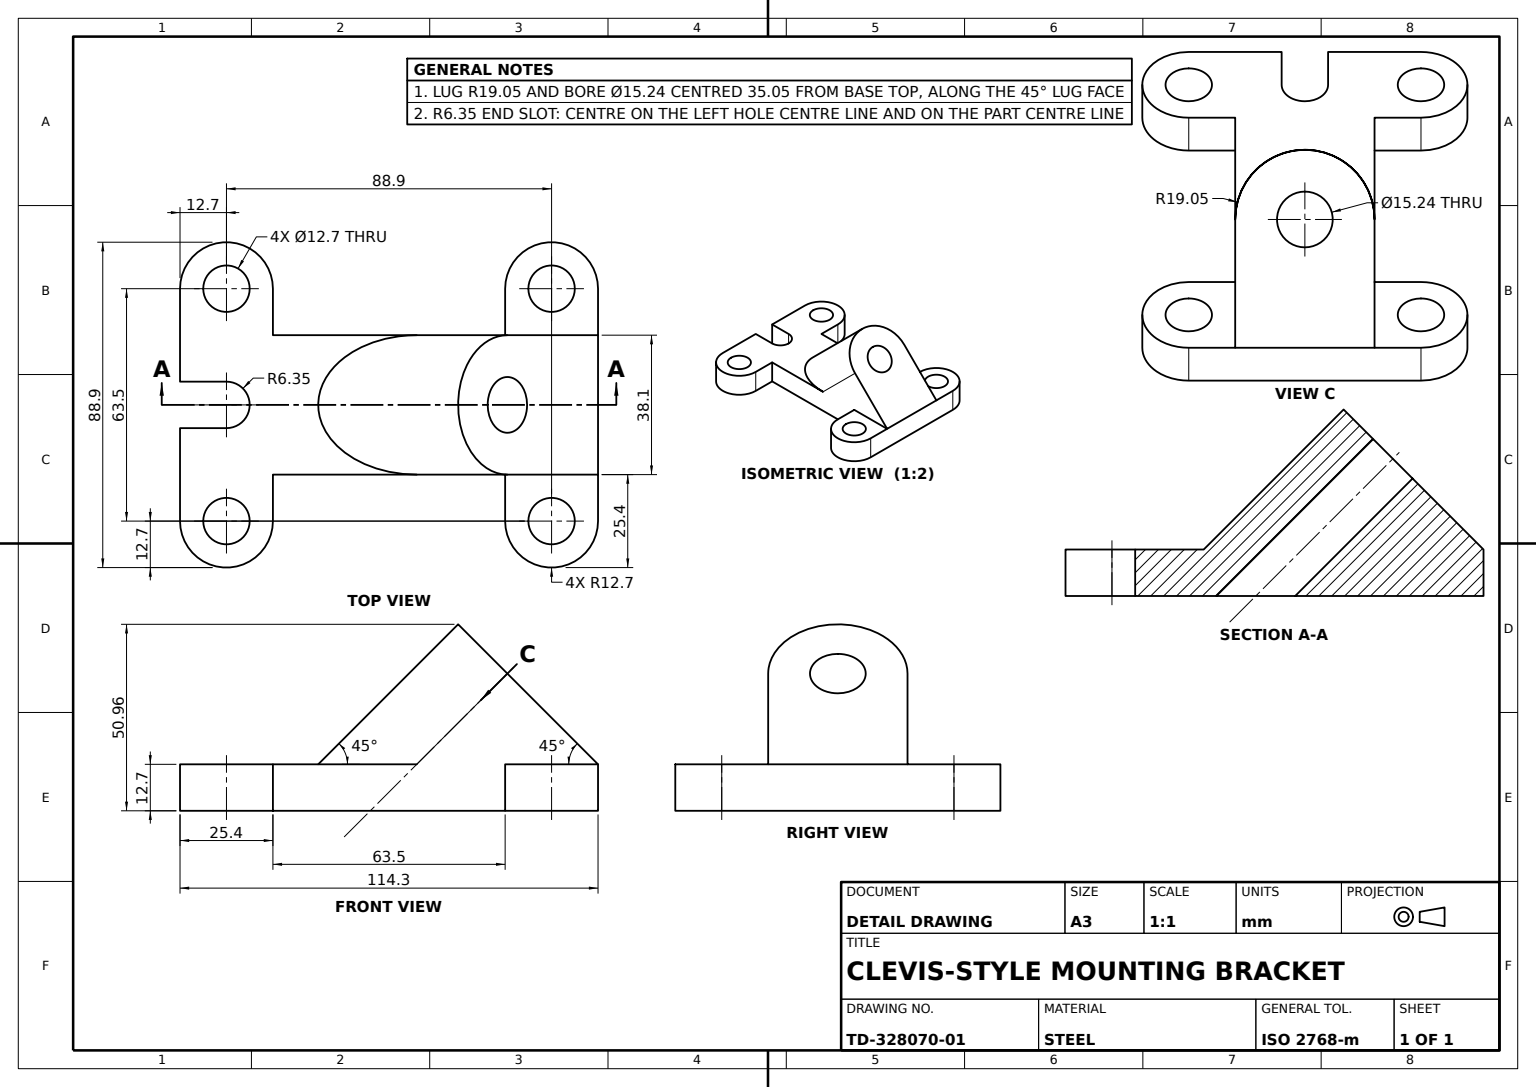
SolidWorks part; units mm, degrees
material "Plain Carbon Steel"
ref_plane "Front Plane" through (0, 0, 0) normal (0, 0, 1) x (1, 0, 0)
ref_plane "Top Plane" through (0, 0, 0) normal (0, 1, 0) x (1, 0, 0)
ref_plane "Right Plane" through (0, 0, 0) normal (1, 0, 0) x (0, 0, -1)
sketch "Base Plate Sketch" plane through (0, 0, 0) normal (0, 1, 0) x (1, 0, 0)
  line L0 (31.75, 0) -> (-31.75, 0) construction
  line L5 (31.75, -12.7) -> (-31.75, -12.7)
  line L6 (31.75, 12.7) -> (-31.75, 12.7)
  line L7 (31.75, -88.9) -> (-31.75, -88.9) construction
  line L8 (31.75, -101.6) -> (-31.75, -101.6)
  line L9 (31.75, -76.2) -> (-31.75, -76.2)
  line L10 (19.05, -44.45) -> (-19.05, -44.45) construction
  line L15 (-19.05, -12.7) -> (19.05, -12.7)
  line L16 (-19.05, -12.7) -> (-19.05, -76.2)
  line L17 (-19.05, -76.2) -> (19.05, -76.2)
  line L18 (19.05, -12.7) -> (19.05, -76.2)
  arc A0 (31.75, -12.7) -> (31.75, 12.7) centre (31.75, 0) ccw
  arc A1 (-31.75, 12.7) -> (-31.75, -12.7) centre (-31.75, 0) ccw
  arc A2 (31.75, -101.6) -> (31.75, -76.2) centre (31.75, -88.9) ccw
  arc A3 (-31.75, -76.2) -> (-31.75, -101.6) centre (-31.75, -88.9) ccw
  point P2 (0, 0)
  point P10 (0, -88.9)
  point P15 (0, -44.45)
  point P16 (-19.05, -12.7)
  point P21 (0, -12.7)
  dimension "D3" = 12.7
  dimension "D1" = 63.5
  dimension "D2" = 88.9
  dimension "D4" = 38.1
extrude "Base Plate" add sketch "Base Plate Sketch" along normal blind 12.7 contours L6 A1 L5 A0 | L18 L5 L16 L9 | L9 A3 L8 A2
sketch "Mounting Holes Sketch" plane through (0, 12.7, 0) normal (0, 1, 0) x (1, 0, 0)
  line L0 (-6.35, 0) -> (-6.35, 12.7)
  line L1 (31.75, 12.7) -> (-31.75, 12.7) construction
  line L2 (-6.35, 12.7) -> (6.35, 12.7)
  line L3 (6.35, 12.7) -> (6.35, 0)
  circle A0 centre (-31.75, 0) radius 6.35
  arc A1 (-6.35, 0) -> (6.35, 0) centre (0, 0) ccw
  circle A2 centre (31.75, 0) radius 6.35
  circle A3 centre (-31.75, -88.9) radius 6.35
  circle A4 centre (31.75, -88.9) radius 6.35
  dimension "D1" = 12.7
extrude "Mounting Holes" cut sketch "Mounting Holes Sketch" against normal through all
ref_plane "Lug Plane 45deg" through (0, 57.15, 57.15) normal (0, 0.7071, 0.7071) x (-1, 0, 0)
sketch "Inclined Lug Sketch" plane through (0, 57.15, 57.15) normal (0, 0.7071, 0.7071) x (-1, 0, 0)
  line L0 (-31.75, 62.8618) -> (31.75, 62.8618) construction
  line L1 (-19.05, 62.8618) -> (19.05, 62.8618)
  line L2 (-19.05, 62.8618) -> (-19.05, 27.8098)
  line L4 (19.05, 62.8618) -> (19.05, 27.8098)
  arc A0 (-19.05, 27.8098) -> (19.05, 27.8098) centre (0, 27.8098) ccw
  dimension "D1" = 35.052
  dimension "D2" = 19.05
extrude "Inclined Lug" add sketch "Inclined Lug Sketch" against normal up to next
sketch "Lug Bore Sketch" plane through (0, 57.15, 57.15) normal (0, 0.7071, 0.7071) x (1, 0, 0)
  circle A0 centre (0, -27.8098) radius 7.62
  dimension "D1" = 15.24
extrude "Lug Bore" cut sketch "Lug Bore Sketch" against normal up to next
